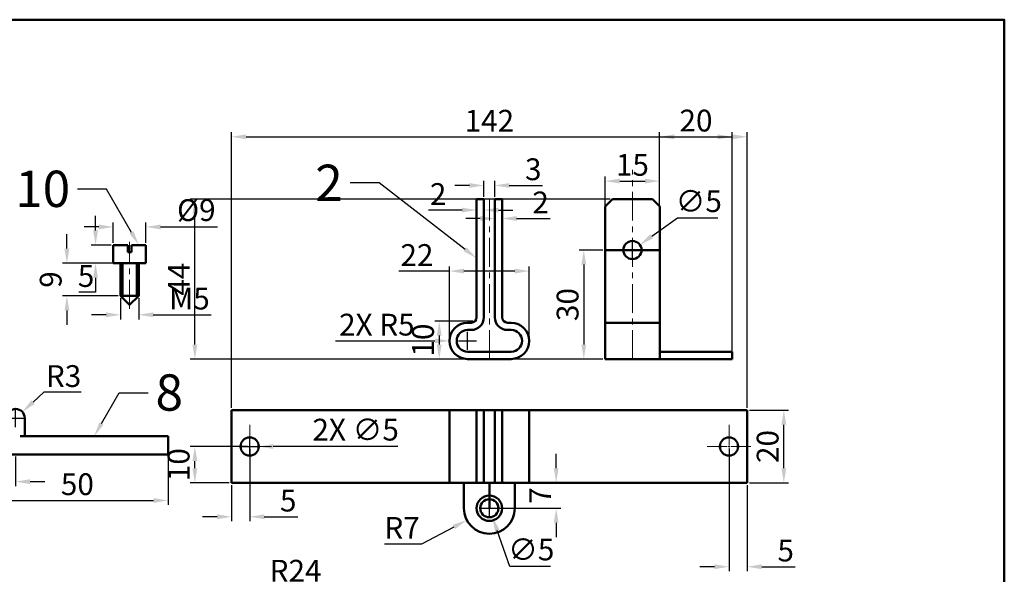
# Model space of a CAD drawing. Units: millimetres. Extents: x 1145 to 1687, y 12 to 400.
# Tile 6 of 6: x 1416 to 1687, y 247 to 400. Entities that reach past the tile are written whole.
import ezdxf
from ezdxf import colors
from ezdxf.entities.mleader import LeaderData, LeaderLine
from ezdxf.math import Vec2, Vec3

# ---------------------------------------------------------------- set-up
doc = ezdxf.new("R2010")
doc.units = ezdxf.units.MM
doc.header["$LTSCALE"] = 0.5
doc.linetypes.add('CENTER', pattern=[50.8, 31.75, -6.35, 6.35, -6.35])
for name, color, linetype, lineweight in [('M-CNTR', 1, 'CENTER', 18), ('M-DIMS', 2, 'Continuous', 25), ('M-OUTL', 7, 'Continuous', 50), ('M-TEXT', 3, 'Continuous', 25)]:
    doc.layers.add(name, color=color, linetype=linetype, lineweight=lineweight)
doc.styles.get("Standard").update_dxf_attribs({"font": 'arial.ttf'})
doc.dimstyles.new('ISO-25', dxfattribs={"dimtxt": 6, "dimasz": 4, "dimexe": 1.25, "dimexo": 0.625, "dimtad": 1, "dimtoh": 1, "dimdec": 0, "dimtxsty": 'Standard', "dimcen": 2.5, "dimadec": 0, "dimazin": 0, "dimtfac": 1, "dimtdec": 0, "dimtofl": 0, "dimtmove": 0, "dimatfit": 3, "dimfxl": 1, "dimarcsym": 0})

# ---------------------------------------------------------------- blocks, each defined once
blk = doc.blocks.new('*D22')
at = {"layer": 'Defpoints', "color": 0, "ltscale": 0.5, "transparency": 16777216}
for p in [(1450.76, 343.09), (1441.76, 338.11), (1450.76, 338.11)]:
    blk.add_point(p, dxfattribs=at)
at = {"layer": 'M-DIMS', "color": 0, "lineweight": -2, "ltscale": 0.5, "transparency": 16777216}
for p, q in [((1437.76, 343.09), (1433.76, 343.09)), ((1441.76, 338.74), (1441.76, 344.34)), ((1450.76, 338.74), (1450.76, 344.34)), ((1454.76, 343.09), (1470.48, 343.09))]:
    blk.add_line(p, q, dxfattribs=at)
at = {"layer": 'M-DIMS', "color": 0, "ltscale": 0.5, "transparency": 16777216}
for points in [[(1437.76, 343.76), (1437.76, 342.42), (1441.76, 343.09)], [(1454.76, 343.76), (1454.76, 342.42), (1450.76, 343.09)]]:
    blk.add_solid(points, dxfattribs=at)
at = {"layer": 'M-DIMS', "color": 0, "ltscale": 0.5, "transparency": 16777216, "insert": (1464.62, 346.94), "char_height": 6, "attachment_point": 5}
blk.add_mtext('%%C9', dxfattribs=at)
blk = doc.blocks.new('*D23')
at = {"layer": 'Defpoints', "color": 0, "ltscale": 0.5, "transparency": 16777216}
for p in [(1441.76, 338.11), (1436.87, 333.11), (1441.76, 333.11)]:
    blk.add_point(p, dxfattribs=at)
at = {"layer": 'M-DIMS', "color": 0, "lineweight": -2, "ltscale": 0.5, "transparency": 16777216}
for p, q in [((1436.87, 342.11), (1436.87, 346.11)), ((1441.14, 338.11), (1435.62, 338.11)), ((1441.14, 333.11), (1435.62, 333.11)), ((1436.87, 329.11), (1436.87, 325.11)), ((1436.87, 325.11), (1432.27, 325.11))]:
    blk.add_line(p, q, dxfattribs=at)
at = {"layer": 'M-DIMS', "color": 0, "ltscale": 0.5, "transparency": 16777216}
for points in [[(1436.2, 342.11), (1437.54, 342.11), (1436.87, 338.11)], [(1436.2, 329.11), (1437.54, 329.11), (1436.87, 333.11)]]:
    blk.add_solid(points, dxfattribs=at)
at = {"layer": 'M-DIMS', "color": 0, "ltscale": 0.5, "transparency": 16777216, "insert": (1434.26, 328.79), "char_height": 6, "attachment_point": 5}
blk.add_mtext('5', dxfattribs=at)
blk = doc.blocks.new('*D24')
at = {"layer": 'Defpoints', "color": 0, "ltscale": 0.5, "transparency": 16777216}
for p in [(1443.76, 324.11), (1448.76, 324.11), (1448.76, 318.9)]:
    blk.add_point(p, dxfattribs=at)
at = {"layer": 'M-DIMS', "color": 0, "lineweight": -2, "ltscale": 0.5, "transparency": 16777216}
for p, q in [((1443.76, 323.49), (1443.76, 317.65)), ((1448.76, 323.49), (1448.76, 317.65)), ((1439.76, 318.9), (1435.76, 318.9)), ((1452.76, 318.9), (1468.7, 318.9))]:
    blk.add_line(p, q, dxfattribs=at)
at = {"layer": 'M-DIMS', "color": 0, "ltscale": 0.5, "transparency": 16777216}
for points in [[(1439.76, 319.57), (1439.76, 318.24), (1443.76, 318.9)], [(1452.76, 319.57), (1452.76, 318.24), (1448.76, 318.9)]]:
    blk.add_solid(points, dxfattribs=at)
at = {"layer": 'M-DIMS', "color": 0, "ltscale": 0.5, "transparency": 16777216, "insert": (1462.73, 322.58), "char_height": 6, "attachment_point": 5}
blk.add_mtext('M5', dxfattribs=at)
blk = doc.blocks.new('*D25')
at = {"layer": 'Defpoints', "color": 0, "ltscale": 0.5, "transparency": 16777216}
for p in [(1443.76, 333.11), (1428.98, 324.11), (1443.76, 324.11)]:
    blk.add_point(p, dxfattribs=at)
at = {"layer": 'M-DIMS', "color": 0, "lineweight": -2, "ltscale": 0.5, "transparency": 16777216}
for p, q in [((1428.98, 337.11), (1428.98, 341.11)), ((1443.14, 333.11), (1427.73, 333.11)), ((1443.14, 324.11), (1427.73, 324.11)), ((1428.98, 320.11), (1428.98, 316.11))]:
    blk.add_line(p, q, dxfattribs=at)
at = {"layer": 'M-DIMS', "color": 0, "ltscale": 0.5, "transparency": 16777216}
for points in [[(1428.31, 337.11), (1429.65, 337.11), (1428.98, 333.11)], [(1428.31, 320.11), (1429.65, 320.11), (1428.98, 324.11)]]:
    blk.add_solid(points, dxfattribs=at)
at = {"layer": 'M-DIMS', "color": 0, "ltscale": 0.5, "transparency": 16777216, "insert": (1425.29, 328.61), "char_height": 6, "attachment_point": 5, "rotation": 90}
blk.add_mtext('9', dxfattribs=at)
blk = doc.blocks.new('*D41')
at = {"layer": 'Defpoints', "color": 0, "ltscale": 0.5, "transparency": 16777216}
for p in [(1406.86, 280.47), (1456.86, 280.47), (1456.86, 267.79)]:
    blk.add_point(p, dxfattribs=at)
at = {"layer": 'M-DIMS', "color": 0, "lineweight": -2, "ltscale": 0.5, "transparency": 16777216}
for p, q in [((1406.86, 279.85), (1406.86, 266.54)), ((1456.86, 279.85), (1456.86, 266.54)), ((1410.86, 267.79), (1452.86, 267.79))]:
    blk.add_line(p, q, dxfattribs=at)
at = {"layer": 'M-DIMS', "color": 0, "ltscale": 0.5, "transparency": 16777216}
for points in [[(1410.86, 268.45), (1410.86, 267.12), (1406.86, 267.79)], [(1452.86, 268.45), (1452.86, 267.12), (1456.86, 267.79)]]:
    blk.add_solid(points, dxfattribs=at)
at = {"layer": 'M-DIMS', "color": 0, "ltscale": 0.5, "transparency": 16777216, "insert": (1431.86, 271.48), "char_height": 6, "attachment_point": 5}
blk.add_mtext('50', dxfattribs=at)
blk = doc.blocks.new('*D42')
at = {"layer": 'Defpoints', "color": 0, "ltscale": 0.5, "transparency": 16777216}
for p in [(1406.86, 280.47), (1414.86, 280.47), (1414.86, 272.97)]:
    blk.add_point(p, dxfattribs=at)
at = {"layer": 'M-DIMS', "color": 0, "lineweight": -2, "ltscale": 0.5, "transparency": 16777216}
for p, q in [((1406.86, 279.85), (1406.86, 271.72)), ((1414.86, 279.85), (1414.86, 271.72)), ((1402.86, 272.97), (1398.86, 272.97)), ((1418.86, 272.97), (1422.86, 272.97))]:
    blk.add_line(p, q, dxfattribs=at)
at = {"layer": 'M-DIMS', "color": 0, "ltscale": 0.5, "transparency": 16777216}
for points in [[(1402.86, 273.63), (1402.86, 272.3), (1406.86, 272.97)], [(1418.86, 273.63), (1418.86, 272.3), (1414.86, 272.97)]]:
    blk.add_solid(points, dxfattribs=at)
at = {"layer": 'M-DIMS', "color": 0, "ltscale": 0.5, "transparency": 16777216, "insert": (1410.86, 276.66), "char_height": 6, "attachment_point": 5}
blk.add_mtext('8', dxfattribs=at)
blk = doc.blocks.new('*D45')
at = {"layer": 'Defpoints', "color": 0, "ltscale": 0.5, "transparency": 16777216}
for p in [(1546.82, 354.5), (1543.82, 350.72), (1546.82, 350.72)]:
    blk.add_point(p, dxfattribs=at)
at = {"layer": 'M-DIMS', "color": 0, "lineweight": -2, "ltscale": 0.5, "transparency": 16777216}
for p, q in [((1543.82, 351.35), (1543.82, 355.75)), ((1546.82, 351.35), (1546.82, 355.75)), ((1539.82, 354.5), (1535.82, 354.5)), ((1550.82, 354.5), (1560, 354.5))]:
    blk.add_line(p, q, dxfattribs=at)
at = {"layer": 'M-DIMS', "color": 0, "ltscale": 0.5, "transparency": 16777216}
for points in [[(1539.82, 355.17), (1539.82, 353.84), (1543.82, 354.5)], [(1550.82, 355.17), (1550.82, 353.84), (1546.82, 354.5)]]:
    blk.add_solid(points, dxfattribs=at)
at = {"layer": 'M-DIMS', "color": 0, "ltscale": 0.5, "transparency": 16777216, "insert": (1557.41, 358.19), "char_height": 6, "attachment_point": 5}
blk.add_mtext('3', dxfattribs=at)
blk = doc.blocks.new('*D46')
at = {"layer": 'Defpoints', "color": 0, "ltscale": 0.5, "transparency": 16777216}
for p in [(1546.82, 350.72), (1548.82, 350.72), (1548.82, 345.41)]:
    blk.add_point(p, dxfattribs=at)
at = {"layer": 'M-DIMS', "color": 0, "lineweight": -2, "ltscale": 0.5, "transparency": 16777216}
for p, q in [((1546.82, 350.1), (1546.82, 344.16)), ((1548.82, 350.1), (1548.82, 344.16)), ((1542.82, 345.41), (1538.82, 345.41)), ((1552.82, 345.41), (1562.04, 345.41))]:
    blk.add_line(p, q, dxfattribs=at)
at = {"layer": 'M-DIMS', "color": 0, "ltscale": 0.5, "transparency": 16777216}
for points in [[(1542.82, 346.08), (1542.82, 344.75), (1546.82, 345.41)], [(1552.82, 346.08), (1552.82, 344.75), (1548.82, 345.41)]]:
    blk.add_solid(points, dxfattribs=at)
at = {"layer": 'M-DIMS', "color": 0, "ltscale": 0.5, "transparency": 16777216, "insert": (1559.43, 349.05), "char_height": 6, "attachment_point": 5}
blk.add_mtext('2', dxfattribs=at)
blk = doc.blocks.new('*D47')
at = {"layer": 'Defpoints', "color": 0, "ltscale": 0.5, "transparency": 16777216}
for p in [(1541.82, 350.72), (1543.82, 350.72), (1543.82, 347.73)]:
    blk.add_point(p, dxfattribs=at)
at = {"layer": 'M-DIMS', "color": 0, "lineweight": -2, "ltscale": 0.5, "transparency": 16777216}
for p, q in [((1541.82, 350.1), (1541.82, 346.48)), ((1543.82, 350.1), (1543.82, 346.48)), ((1537.82, 347.73), (1528.6, 347.73)), ((1547.82, 347.73), (1551.82, 347.73))]:
    blk.add_line(p, q, dxfattribs=at)
at = {"layer": 'M-DIMS', "color": 0, "ltscale": 0.5, "transparency": 16777216}
for points in [[(1537.82, 348.39), (1537.82, 347.06), (1541.82, 347.73)], [(1547.82, 348.39), (1547.82, 347.06), (1543.82, 347.73)]]:
    blk.add_solid(points, dxfattribs=at)
at = {"layer": 'M-DIMS', "color": 0, "ltscale": 0.5, "transparency": 16777216, "insert": (1531.21, 351.36), "char_height": 6, "attachment_point": 5}
blk.add_mtext('2', dxfattribs=at)
blk = doc.blocks.new('*D48')
at = {"layer": 'Defpoints', "color": 0, "ltscale": 0.5, "transparency": 16777216}
for p in [(1577.22, 336.72), (1571.33, 306.72), (1577.22, 306.72)]:
    blk.add_point(p, dxfattribs=at)
at = {"layer": 'M-DIMS', "color": 0, "lineweight": -2, "ltscale": 0.5, "transparency": 16777216}
for p, q in [((1576.6, 336.72), (1570.08, 336.72)), ((1571.33, 332.72), (1571.33, 310.72)), ((1576.6, 306.72), (1570.08, 306.72))]:
    blk.add_line(p, q, dxfattribs=at)
at = {"layer": 'M-DIMS', "color": 0, "ltscale": 0.5, "transparency": 16777216}
for points in [[(1570.66, 332.72), (1571.99, 332.72), (1571.33, 336.72)], [(1570.66, 310.72), (1571.99, 310.72), (1571.33, 306.72)]]:
    blk.add_solid(points, dxfattribs=at)
at = {"layer": 'M-DIMS', "color": 0, "ltscale": 0.5, "transparency": 16777216, "insert": (1567.64, 321.72), "char_height": 6, "attachment_point": 5, "rotation": 90}
blk.add_mtext('30', dxfattribs=at)
blk = doc.blocks.new('*D49')
at = {"layer": 'Defpoints', "color": 0, "ltscale": 0.5, "transparency": 16777216}
for p in [(1541.38, 317.16), (1531.52, 306.72), (1541.38, 306.72)]:
    blk.add_point(p, dxfattribs=at)
at = {"layer": 'M-DIMS', "color": 0, "lineweight": -2, "ltscale": 0.5, "transparency": 16777216}
for p, q in [((1540.76, 317.16), (1530.27, 317.16)), ((1531.52, 313.16), (1531.52, 310.72)), ((1540.76, 306.72), (1530.27, 306.72))]:
    blk.add_line(p, q, dxfattribs=at)
at = {"layer": 'M-DIMS', "color": 0, "ltscale": 0.5, "transparency": 16777216}
for points in [[(1530.85, 313.16), (1532.19, 313.16), (1531.52, 317.16)], [(1530.85, 310.72), (1532.19, 310.72), (1531.52, 306.72)]]:
    blk.add_solid(points, dxfattribs=at)
at = {"layer": 'M-DIMS', "color": 0, "ltscale": 0.5, "transparency": 16777216, "insert": (1527.83, 311.94), "char_height": 6, "attachment_point": 5, "rotation": 90}
blk.add_mtext('10', dxfattribs=at)
blk = doc.blocks.new('*D50')
at = {"layer": 'Defpoints', "color": 0, "ltscale": 0.5, "transparency": 16777216}
for p in [(1556.32, 330.94), (1534.32, 311.72), (1556.32, 311.72)]:
    blk.add_point(p, dxfattribs=at)
at = {"layer": 'M-DIMS', "color": 0, "lineweight": -2, "ltscale": 0.5, "transparency": 16777216}
for p, q in [((1534.32, 330.94), (1520.43, 330.94)), ((1534.32, 312.35), (1534.32, 332.19)), ((1552.32, 330.94), (1538.32, 330.94)), ((1556.32, 312.35), (1556.32, 332.19))]:
    blk.add_line(p, q, dxfattribs=at)
at = {"layer": 'M-DIMS', "color": 0, "ltscale": 0.5, "transparency": 16777216}
for points in [[(1538.32, 331.6), (1538.32, 330.27), (1534.32, 330.94)], [(1552.32, 331.6), (1552.32, 330.27), (1556.32, 330.94)]]:
    blk.add_solid(points, dxfattribs=at)
at = {"layer": 'M-DIMS', "color": 0, "ltscale": 0.5, "transparency": 16777216, "insert": (1525.38, 334.57), "char_height": 6, "attachment_point": 5}
blk.add_mtext('22', dxfattribs=at)
blk = doc.blocks.new('*D51')
at = {"layer": 'Defpoints', "color": 0, "ltscale": 0.5, "transparency": 16777216}
for p in [(1592.22, 355.71), (1577.22, 342.72), (1592.22, 342.72)]:
    blk.add_point(p, dxfattribs=at)
at = {"layer": 'M-DIMS', "color": 0, "lineweight": -2, "ltscale": 0.5, "transparency": 16777216}
for p, q in [((1577.22, 343.35), (1577.22, 356.96)), ((1581.22, 355.71), (1588.22, 355.71)), ((1592.22, 343.35), (1592.22, 356.96))]:
    blk.add_line(p, q, dxfattribs=at)
at = {"layer": 'M-DIMS', "color": 0, "ltscale": 0.5, "transparency": 16777216}
for points in [[(1581.22, 356.38), (1581.22, 355.05), (1577.22, 355.71)], [(1588.22, 356.38), (1588.22, 355.05), (1592.22, 355.71)]]:
    blk.add_solid(points, dxfattribs=at)
at = {"layer": 'M-DIMS', "color": 0, "ltscale": 0.5, "transparency": 16777216, "insert": (1584.72, 359.4), "char_height": 6, "attachment_point": 5}
blk.add_mtext('15', dxfattribs=at)
blk = doc.blocks.new('*D52')
at = {"layer": 'Defpoints', "color": 0, "ltscale": 0.5, "transparency": 16777216}
for p in [(1586.76, 338.17), (1582.69, 335.27)]:
    blk.add_point(p, dxfattribs=at)
at = {"layer": 'M-DIMS', "color": 0, "lineweight": -2, "ltscale": 0.5, "transparency": 16777216}
for p, q in [((1597.11, 345.54), (1590.02, 340.49)), ((1608.24, 345.54), (1597.11, 345.54)), ((1584.72, 334.22), (1584.72, 339.22)), ((1582.22, 336.72), (1587.22, 336.72))]:
    blk.add_line(p, q, dxfattribs=at)
at = {"layer": 'M-DIMS', "color": 0, "ltscale": 0.5, "transparency": 16777216}
blk.add_solid([(1589.63, 341.04), (1590.4, 339.95), (1586.76, 338.17)], dxfattribs=at)
at = {"layer": 'M-DIMS', "color": 0, "ltscale": 0.5, "transparency": 16777216, "insert": (1602.99, 349.4), "char_height": 6, "attachment_point": 5}
blk.add_mtext('∅5', dxfattribs=at)
blk = doc.blocks.new('*U56')
at = {"layer": 'M-CNTR', "color": 0, "transparency": 16777216}
for p, q in [((0, 0.5), (0, 6)), ((-6, 0), (-0.5, 0)), ((0.5, 0), (6, 0)), ((0, -6), (0, -0.5))]:
    blk.add_line(p, q, dxfattribs=at)
at = {"layer": 'M-CNTR', "color": 0, "linetype": 'Continuous', "transparency": 16777216}
for p, q in [((-0.25, 0), (0.25, 0)), ((0, -0.25), (0, 0.25))]:
    blk.add_line(p, q, dxfattribs=at)
blk = doc.blocks.new('*U57')
at = {"layer": 'M-CNTR', "color": 0, "transparency": 16777216}
for p, q in [((0, 0.5), (0, 6)), ((-6, 0), (-0.5, 0)), ((0.5, 0), (6, 0)), ((0, -6), (0, -0.5))]:
    blk.add_line(p, q, dxfattribs=at)
at = {"layer": 'M-CNTR', "color": 0, "linetype": 'Continuous', "transparency": 16777216}
for p, q in [((-0.25, 0), (0.25, 0)), ((0, -0.25), (0, 0.25))]:
    blk.add_line(p, q, dxfattribs=at)
blk = doc.blocks.new('*D58')
at = {"layer": 'Defpoints', "color": 0, "ltscale": 0.5, "transparency": 16777216}
for p in [(1479.32, 282.64), (1474.32, 272.64), (1479.32, 263.29)]:
    blk.add_point(p, dxfattribs=at)
at = {"layer": 'M-DIMS', "color": 0, "lineweight": -2, "ltscale": 0.5, "transparency": 16777216}
for p, q in [((1479.32, 282.02), (1479.32, 262.04)), ((1474.32, 272.02), (1474.32, 262.04)), ((1470.32, 263.29), (1466.32, 263.29)), ((1483.32, 263.29), (1492.55, 263.29))]:
    blk.add_line(p, q, dxfattribs=at)
at = {"layer": 'M-DIMS', "color": 0, "ltscale": 0.5, "transparency": 16777216}
for points in [[(1470.32, 263.96), (1470.32, 262.62), (1474.32, 263.29)], [(1483.32, 263.96), (1483.32, 262.62), (1479.32, 263.29)]]:
    blk.add_solid(points, dxfattribs=at)
at = {"layer": 'M-DIMS', "color": 0, "ltscale": 0.5, "transparency": 16777216, "insert": (1489.93, 266.97), "char_height": 6, "attachment_point": 5}
blk.add_mtext('5', dxfattribs=at)
blk = doc.blocks.new('*D59')
at = {"layer": 'Defpoints', "color": 0, "ltscale": 0.5, "transparency": 16777216}
for p in [(1414.86, 290.47), (1416.7, 292.16)]:
    blk.add_point(p, dxfattribs=at)
at = {"layer": 'M-DIMS', "color": 0, "lineweight": -2, "ltscale": 0.5, "transparency": 16777216}
for p, q in [((1422.6, 297.56), (1419.65, 294.86)), ((1432.9, 297.56), (1422.6, 297.56)), ((1414.86, 287.97), (1414.86, 292.97)), ((1412.36, 290.47), (1417.36, 290.47))]:
    blk.add_line(p, q, dxfattribs=at)
at = {"layer": 'M-DIMS', "color": 0, "ltscale": 0.5, "transparency": 16777216}
blk.add_solid([(1419.2, 295.35), (1420.1, 294.37), (1416.7, 292.16)], dxfattribs=at)
at = {"layer": 'M-DIMS', "color": 0, "ltscale": 0.5, "transparency": 16777216, "insert": (1428.06, 301.25), "char_height": 6, "attachment_point": 5}
blk.add_mtext('R3', dxfattribs=at)
blk = doc.blocks.new('*D66')
at = {"layer": 'Defpoints', "color": 0, "ltscale": 0.5, "transparency": 16777216}
for p in [(1545.32, 272.64), (1545.32, 265.64), (1563.72, 265.64)]:
    blk.add_point(p, dxfattribs=at)
at = {"layer": 'M-DIMS', "color": 0, "lineweight": -2, "ltscale": 0.5, "transparency": 16777216}
for p, q in [((1563.72, 276.64), (1563.72, 280.64)), ((1545.95, 272.64), (1564.97, 272.64)), ((1545.95, 265.64), (1564.97, 265.64)), ((1563.72, 261.64), (1563.72, 257.64))]:
    blk.add_line(p, q, dxfattribs=at)
at = {"layer": 'M-DIMS', "color": 0, "ltscale": 0.5, "transparency": 16777216}
for points in [[(1563.05, 276.64), (1564.38, 276.64), (1563.72, 272.64)], [(1563.05, 261.64), (1564.38, 261.64), (1563.72, 265.64)]]:
    blk.add_solid(points, dxfattribs=at)
at = {"layer": 'M-DIMS', "color": 0, "ltscale": 0.5, "transparency": 16777216, "insert": (1560.09, 269.14), "char_height": 6, "attachment_point": 5, "rotation": 90}
blk.add_mtext('7', dxfattribs=at)
blk = doc.blocks.new('*D67')
at = {"layer": 'Defpoints', "color": 0, "ltscale": 0.5, "transparency": 16777216}
for p in [(1545.32, 265.64), (1539.13, 262.37)]:
    blk.add_point(p, dxfattribs=at)
at = {"layer": 'M-DIMS', "color": 0, "lineweight": -2, "ltscale": 0.5, "transparency": 16777216}
for p, q in [((1545.32, 263.14), (1545.32, 268.14)), ((1542.82, 265.64), (1547.82, 265.64)), ((1526.75, 255.84), (1535.59, 260.51)), ((1516.45, 255.84), (1526.75, 255.84))]:
    blk.add_line(p, q, dxfattribs=at)
at = {"layer": 'M-DIMS', "color": 0, "ltscale": 0.5, "transparency": 16777216}
blk.add_solid([(1535.28, 261.09), (1535.9, 259.92), (1539.13, 262.37)], dxfattribs=at)
at = {"layer": 'M-DIMS', "color": 0, "ltscale": 0.5, "transparency": 16777216, "insert": (1521.29, 259.46), "char_height": 6, "attachment_point": 5}
blk.add_mtext('R7', dxfattribs=at)
blk = doc.blocks.new('*D68')
at = {"layer": 'Defpoints', "color": 0, "ltscale": 0.5, "transparency": 16777216}
for p in [(1544.49, 268), (1546.16, 263.28)]:
    blk.add_point(p, dxfattribs=at)
at = {"layer": 'M-DIMS', "color": 0, "lineweight": -2, "ltscale": 0.5, "transparency": 16777216}
for p, q in [((1545.32, 263.14), (1545.32, 268.14)), ((1542.82, 265.64), (1547.82, 265.64)), ((1550.99, 249.65), (1547.49, 259.51)), ((1562.12, 249.65), (1550.99, 249.65))]:
    blk.add_line(p, q, dxfattribs=at)
at = {"layer": 'M-DIMS', "color": 0, "ltscale": 0.5, "transparency": 16777216}
blk.add_solid([(1548.12, 259.74), (1546.86, 259.29), (1546.16, 263.28)], dxfattribs=at)
at = {"layer": 'M-DIMS', "color": 0, "ltscale": 0.5, "transparency": 16777216, "insert": (1556.86, 253.51), "char_height": 6, "attachment_point": 5}
blk.add_mtext('∅5', dxfattribs=at)
blk = doc.blocks.new('CONTACT-CLIP')
at = {"ltscale": 0.5}
for p, q in [((7.5, 11.5), (7.5, 44)), ((7.5, 44), (9.5, 44)), ((9.5, 11.5), (9.5, 44)), ((12.5, 11.5), (12.5, 44)), ((12.5, 44), (14.5, 44)), ((14.5, 11.5), (14.5, 44)), ((5, 10), (6, 10)), ((5, 2), (17, 2)), ((5, 0), (17, 0))]:
    blk.add_line(p, q, dxfattribs=at)
for centre, radius, start, end in [((6, 11.5), 1.5, 270, 0), ((6, 11.5), 3.5, 270, 0), ((16, 11.5), 3.5, 180, 270), ((16, 11.5), 1.5, 180, 270), ((5, 5), 5, 90, 270), ((17, 5), 5, 270, 90), ((5, 5), 3, 90, 270), ((17, 5), 3, 270, 90)]:
    blk.add_arc(centre, radius, start, end, dxfattribs=at)
for points in [[(16, 10), (16.33, 10), (16.67, 10), (17, 10)], [(6, 8), (5.67, 8), (5.33, 8), (5, 8)], [(16, 8), (16.33, 8), (16.67, 8), (17, 8)]]:
    blk.add_open_spline(points, degree=3)
blk = doc.blocks.new('SCREW-HEAD')
at = {"ltscale": 0.5}
for p, q in [((0, 5), (4, 5)), ((0, 0), (0, 5)), ((4, 5), (4, 3)), ((4, 3), (5, 3)), ((5, 5), (5, 3)), ((5, 5), (9, 5)), ((9, 5), (9, 0)), ((9, 0), (0, 0))]:
    blk.add_line(p, q, dxfattribs=at)
blk = doc.blocks.new('TERMINAL-LUG-END')
at = {"ltscale": 0.5}
for p, q in [((0, 7), (0, 14)), ((14, 7), (14, 14))]:
    blk.add_line(p, q, dxfattribs=at)
blk.add_arc((7, 7), 7, 180, 0, dxfattribs=at)
blk = doc.blocks.new('*D90')
at = {"layer": 'Defpoints', "color": 0, "ltscale": 0.5, "transparency": 16777216}
for p in [(1616.32, 367.9), (1474.32, 292.64), (1616.32, 292.64)]:
    blk.add_point(p, dxfattribs=at)
at = {"layer": 'M-DIMS', "color": 0, "lineweight": -2, "ltscale": 0.5, "transparency": 16777216}
for p, q in [((1474.32, 293.27), (1474.32, 369.15)), ((1616.32, 293.27), (1616.32, 369.15)), ((1478.32, 367.9), (1612.32, 367.9))]:
    blk.add_line(p, q, dxfattribs=at)
at = {"layer": 'M-DIMS', "color": 0, "ltscale": 0.5, "transparency": 16777216}
for points in [[(1478.32, 368.57), (1478.32, 367.23), (1474.32, 367.9)], [(1612.32, 368.57), (1612.32, 367.23), (1616.32, 367.9)]]:
    blk.add_solid(points, dxfattribs=at)
at = {"layer": 'M-DIMS', "color": 0, "ltscale": 0.5, "transparency": 16777216, "insert": (1545.32, 371.54), "char_height": 6, "attachment_point": 5}
blk.add_mtext('142', dxfattribs=at)
blk = doc.blocks.new('*D91')
at = {"layer": 'Defpoints', "color": 0, "ltscale": 0.5, "transparency": 16777216}
for p in [(1616.32, 292.64), (1626.42, 292.64), (1616.32, 272.64)]:
    blk.add_point(p, dxfattribs=at)
at = {"layer": 'M-DIMS', "color": 0, "lineweight": -2, "ltscale": 0.5, "transparency": 16777216}
for p, q in [((1616.95, 292.64), (1627.67, 292.64)), ((1626.42, 276.64), (1626.42, 288.64)), ((1616.95, 272.64), (1627.67, 272.64))]:
    blk.add_line(p, q, dxfattribs=at)
at = {"layer": 'M-DIMS', "color": 0, "ltscale": 0.5, "transparency": 16777216}
for points in [[(1625.75, 288.64), (1627.09, 288.64), (1626.42, 292.64)], [(1625.75, 276.64), (1627.09, 276.64), (1626.42, 272.64)]]:
    blk.add_solid(points, dxfattribs=at)
at = {"layer": 'M-DIMS', "color": 0, "ltscale": 0.5, "transparency": 16777216, "insert": (1622.73, 282.64), "char_height": 6, "attachment_point": 5, "rotation": 90}
blk.add_mtext('20', dxfattribs=at)
blk = doc.blocks.new('*D92')
at = {"layer": 'Defpoints', "color": 0, "ltscale": 0.5, "transparency": 16777216}
for p in [(1611.32, 282.64), (1616.32, 272.64), (1616.32, 249.54)]:
    blk.add_point(p, dxfattribs=at)
at = {"layer": 'M-DIMS', "color": 0, "lineweight": -2, "ltscale": 0.5, "transparency": 16777216}
for p, q in [((1611.32, 282.02), (1611.32, 248.29)), ((1616.32, 272.02), (1616.32, 248.29)), ((1607.32, 249.54), (1603.32, 249.54)), ((1620.32, 249.54), (1629.55, 249.54))]:
    blk.add_line(p, q, dxfattribs=at)
at = {"layer": 'M-DIMS', "color": 0, "ltscale": 0.5, "transparency": 16777216}
for points in [[(1607.32, 250.21), (1607.32, 248.87), (1611.32, 249.54)], [(1620.32, 250.21), (1620.32, 248.87), (1616.32, 249.54)]]:
    blk.add_solid(points, dxfattribs=at)
at = {"layer": 'M-DIMS', "color": 0, "ltscale": 0.5, "transparency": 16777216, "insert": (1626.93, 253.22), "char_height": 6, "attachment_point": 5}
blk.add_mtext('5', dxfattribs=at)
blk = doc.blocks.new('*D93')
at = {"layer": 'Defpoints', "color": 0, "ltscale": 0.5, "transparency": 16777216}
for p in [(1464.22, 282.64), (1479.32, 282.64), (1474.32, 272.64)]:
    blk.add_point(p, dxfattribs=at)
at = {"layer": 'M-DIMS', "color": 0, "lineweight": -2, "ltscale": 0.5, "transparency": 16777216}
for p, q in [((1478.7, 282.64), (1462.97, 282.64)), ((1464.22, 276.64), (1464.22, 278.64)), ((1473.7, 272.64), (1462.97, 272.64))]:
    blk.add_line(p, q, dxfattribs=at)
at = {"layer": 'M-DIMS', "color": 0, "ltscale": 0.5, "transparency": 16777216}
for points in [[(1463.55, 278.64), (1464.89, 278.64), (1464.22, 282.64)], [(1463.55, 276.64), (1464.89, 276.64), (1464.22, 272.64)]]:
    blk.add_solid(points, dxfattribs=at)
at = {"layer": 'M-DIMS', "color": 0, "ltscale": 0.5, "transparency": 16777216, "insert": (1460.53, 277.64), "char_height": 6, "attachment_point": 5, "rotation": 90}
blk.add_mtext('10', dxfattribs=at)
blk = doc.blocks.new('*D94')
at = {"layer": 'Defpoints', "color": 0, "ltscale": 0.5, "transparency": 16777216}
for p in [(1464.22, 350.72), (1579.22, 350.72), (1577.22, 306.72)]:
    blk.add_point(p, dxfattribs=at)
at = {"layer": 'M-DIMS', "color": 0, "lineweight": -2, "ltscale": 0.5, "transparency": 16777216}
for p, q in [((1578.6, 350.72), (1462.97, 350.72)), ((1464.22, 310.72), (1464.22, 346.72)), ((1576.6, 306.72), (1462.97, 306.72))]:
    blk.add_line(p, q, dxfattribs=at)
at = {"layer": 'M-DIMS', "color": 0, "ltscale": 0.5, "transparency": 16777216}
for points in [[(1463.55, 346.72), (1464.89, 346.72), (1464.22, 350.72)], [(1463.55, 310.72), (1464.89, 310.72), (1464.22, 306.72)]]:
    blk.add_solid(points, dxfattribs=at)
at = {"layer": 'M-DIMS', "color": 0, "ltscale": 0.5, "transparency": 16777216, "insert": (1460.6, 328.72), "char_height": 6, "attachment_point": 5, "rotation": 90}
blk.add_mtext('44', dxfattribs=at)
blk = doc.blocks.new('*D95')
at = {"layer": 'Defpoints', "color": 0, "ltscale": 0.5, "transparency": 16777216}
for p in [(1612.22, 367.9), (1592.22, 306.72), (1612.22, 306.72)]:
    blk.add_point(p, dxfattribs=at)
at = {"layer": 'M-DIMS', "color": 0, "lineweight": -2, "ltscale": 0.5, "transparency": 16777216}
for p, q in [((1592.22, 307.35), (1592.22, 369.15)), ((1612.22, 307.35), (1612.22, 369.15)), ((1596.22, 367.9), (1608.22, 367.9))]:
    blk.add_line(p, q, dxfattribs=at)
at = {"layer": 'M-DIMS', "color": 0, "ltscale": 0.5, "transparency": 16777216}
for points in [[(1596.22, 368.57), (1596.22, 367.23), (1592.22, 367.9)], [(1608.22, 368.57), (1608.22, 367.23), (1612.22, 367.9)]]:
    blk.add_solid(points, dxfattribs=at)
at = {"layer": 'M-DIMS', "color": 0, "ltscale": 0.5, "transparency": 16777216, "insert": (1602.22, 371.59), "char_height": 6, "attachment_point": 5}
blk.add_mtext('20', dxfattribs=at)
blk = doc.blocks.new('*D115')
at = {"layer": 'Defpoints', "color": 0, "ltscale": 0.5, "transparency": 16777216}
for p in [(1476.82, 282.64), (1481.82, 282.64)]:
    blk.add_point(p, dxfattribs=at)
at = {"layer": 'M-DIMS', "color": 0, "lineweight": -2, "ltscale": 0.5, "transparency": 16777216}
for p, q in [((1479.32, 280.14), (1479.32, 285.14)), ((1476.82, 282.64), (1481.82, 282.64)), ((1496.28, 282.64), (1485.82, 282.64)), ((1520.09, 282.64), (1496.28, 282.64))]:
    blk.add_line(p, q, dxfattribs=at)
at = {"layer": 'M-DIMS', "color": 0, "ltscale": 0.5, "transparency": 16777216}
blk.add_solid([(1485.82, 283.31), (1485.82, 281.97), (1481.82, 282.64)], dxfattribs=at)
at = {"layer": 'M-DIMS', "color": 0, "ltscale": 0.5, "transparency": 16777216, "insert": (1508.5, 286.5), "char_height": 6, "attachment_point": 5}
blk.add_mtext('2X ∅5', dxfattribs=at)
blk = doc.blocks.new('*D116')
at = {"layer": 'Defpoints', "color": 0, "ltscale": 0.5, "transparency": 16777216}
for p in [(1534.32, 311.72), (1539.32, 311.72)]:
    blk.add_point(p, dxfattribs=at)
at = {"layer": 'M-DIMS', "color": 0, "lineweight": -2, "ltscale": 0.5, "transparency": 16777216}
for p, q in [((1539.32, 309.22), (1539.32, 314.22)), ((1502.98, 311.72), (1526.32, 311.72)), ((1526.32, 311.72), (1530.32, 311.72)), ((1536.82, 311.72), (1541.82, 311.72))]:
    blk.add_line(p, q, dxfattribs=at)
at = {"layer": 'M-DIMS', "color": 0, "ltscale": 0.5, "transparency": 16777216}
blk.add_solid([(1530.32, 312.39), (1530.32, 311.06), (1534.32, 311.72)], dxfattribs=at)
at = {"layer": 'M-DIMS', "color": 0, "ltscale": 0.5, "transparency": 16777216, "insert": (1514.34, 315.41), "char_height": 6, "attachment_point": 5}
blk.add_mtext('2X R5', dxfattribs=at)
blk = doc.blocks.new('*D119')
at = {"layer": 'Defpoints', "color": 0, "ltscale": 0.5, "transparency": 16777216}
for p in [(1499.73, 229.62), (1499.73, 205.62)]:
    blk.add_point(p, dxfattribs=at)
at = {"layer": 'M-DIMS', "color": 0, "lineweight": -2, "ltscale": 0.5, "transparency": 16777216}
for p, q in [((1484.79, 244.02), (1499.73, 244.02)), ((1499.73, 244.02), (1499.73, 233.62)), ((1499.73, 203.12), (1499.73, 208.12)), ((1497.23, 205.62), (1502.23, 205.62))]:
    blk.add_line(p, q, dxfattribs=at)
at = {"layer": 'M-DIMS', "color": 0, "ltscale": 0.5, "transparency": 16777216}
blk.add_solid([(1500.4, 233.62), (1499.07, 233.62), (1499.73, 229.62)], dxfattribs=at)
at = {"layer": 'M-DIMS', "color": 0, "ltscale": 0.5, "transparency": 16777216, "insert": (1491.95, 247.66), "char_height": 6, "attachment_point": 5}
blk.add_mtext('R24', dxfattribs=at)

msp = doc.modelspace()

# ---------------------------------------------------------------- linework, layer by layer
at = {"layer": 'M-CNTR', "ltscale": 0.5}
for p, q in [((1584.7228, 306.7236), (1584.7228, 358.8009)), ((1545.3206, 306.7236), (1545.3206, 350.7236)), ((1446.2604, 320.5579), (1446.2604, 338.9798))]:
    msp.add_line(p, q, dxfattribs=at)
at = {"layer": 'M-OUTL', "ltscale": 0.5}
for p, q in [((1577.2228, 348.7236), (1579.2228, 350.7236)), ((1579.2228, 350.7236), (1590.2228, 350.7236)), ((1592.2228, 348.7236), (1590.2228, 350.7236)), ((1577.2228, 336.7236), (1577.2228, 348.7236)), ((1592.2228, 348.7236), (1592.2228, 336.7236)), ((1592.2228, 336.7236), (1577.2228, 336.7236)), ((1577.2228, 336.7236), (1577.2228, 306.7236)), ((1592.2228, 306.7236), (1592.2228, 336.7236)), ((1443.7604, 333.1137), (1443.7604, 324.1137)), ((1444.2604, 333.1137), (1444.2604, 324.1137)), ((1448.2604, 333.1137), (1448.2604, 324.1137)), ((1448.7604, 333.1137), (1448.7604, 324.1137)), ((1448.7604, 324.1137), (1443.7604, 324.1137)), ((1443.7604, 324.1137), (1446.2604, 321.6152)), ((1448.7604, 324.1137), (1446.2604, 321.6152)), ((1577.2228, 316.7236), (1592.2228, 316.7236)), ((1577.2228, 306.7236), (1592.2228, 306.7236)), ((1612.2228, 308.7236), (1592.2228, 308.7236)), ((1592.2228, 306.7236), (1612.2228, 306.7236)), ((1612.2228, 306.7236), (1612.2228, 308.7236)), ((1417.3568, 290.4724), (1417.3568, 285.4724)), ((1534.3206, 292.6401), (1474.3206, 292.6401)), ((1474.3206, 292.6401), (1474.3206, 272.6401)), ((1534.3206, 292.6401), (1534.3206, 272.6401)), ((1556.3206, 292.6401), (1534.3206, 292.6401)), ((1541.8206, 292.6401), (1541.8206, 272.6401)), ((1543.8206, 292.6401), (1543.8206, 272.6401)), ((1546.8206, 292.6401), (1546.8206, 272.6401)), ((1548.8206, 292.6401), (1548.8206, 272.6401)), ((1556.3206, 292.6401), (1556.3206, 272.6401)), ((1556.3206, 292.6401), (1616.3206, 292.6401)), ((1616.3206, 292.6401), (1616.3206, 272.6401)), ((1456.8568, 285.4724), (1416.1068, 285.4724)), ((1456.8568, 280.4724), (1456.8568, 285.4724)), ((1406.8568, 280.4724), (1456.8568, 280.4724)), ((1474.3206, 272.6401), (1534.3206, 272.6401)), ((1556.3206, 272.6401), (1534.3206, 272.6401)), ((1545.3206, 272.6401), (1545.3206, 265.6401)), ((1616.3206, 272.6401), (1556.3206, 272.6401))]:
    msp.add_line(p, q, dxfattribs=at)
msp.add_lwpolyline([(1145.3327, 400.1417), (1687.1285, 400.1417), (1687.1285, 12.2645), (1145.3327, 12.2645)], close=True, dxfattribs=at)
for centre, radius in [((1584.7228, 336.7236), 2.5), ((1479.3206, 282.6401), 2.5), ((1611.3206, 282.6401), 2.5), ((1545.3206, 265.6401), 3.5), ((1545.3206, 265.6401), 2.5)]:
    msp.add_circle(centre, radius, dxfattribs=at)
msp.add_arc((1414.8568, 290.4724), 2.5, 0, 180, dxfattribs=at)

# ---------------------------------------------------------------- block references
at = {"layer": 'M-CNTR'}
for name, p in [('*U57', (1479.3206, 282.6401)), ('*U56', (1611.3206, 282.6401))]:
    msp.add_blockref(name, p, dxfattribs=at)
at = {"layer": 'M-OUTL'}
for name, p in [('CONTACT-CLIP', (1534.321, 306.724)), ('SCREW-HEAD', (1441.76, 333.114)), ('TERMINAL-LUG-END', (1538.321, 258.64))]:
    msp.add_blockref(name, p, dxfattribs=at)

# ---------------------------------------------------------------- dimensions: what is measured, and where the dimension line sits
at = {"layer": 'M-DIMS', "ltscale": 0.5}
for base, p1, p2, override, picture, middle in [((1616.3206, 367.9009), (1474.3206, 292.6401), (1616.3206, 292.6401), {"dimdec": 0, "dimlfac": 1, "dimrnd": 0, "dimzin": 0, "dimdsep": 46, "dimlunit": 2}, '*D90', (1545.3206, 371.5382)), ((1612.2228, 367.9009), (1592.2228, 306.7236), (1612.2228, 306.7236), {"dimdec": 0, "dimlfac": 1, "dimrnd": 0, "dimzin": 0, "dimdsep": 46, "dimlunit": 2}, '*D95', (1602.2228, 371.5893)), ((1592.2228, 355.714), (1577.2228, 342.7236), (1592.2228, 342.7236), {"dimclrd": 0, "dimclre": 0, "dimclrt": 0}, '*D51', (1584.7228, 359.4024)), ((1546.8206, 354.5041), (1543.8206, 350.7236), (1546.8206, 350.7236), {"dimclrd": 0, "dimclre": 0, "dimclrt": 0}, '*D45', (1557.4101, 358.1946)), ((1548.8206, 345.4149), (1546.8206, 350.7236), (1548.8206, 350.7236), {"dimclrd": 0, "dimclre": 0, "dimclrt": 0}, '*D46', (1559.4326, 349.0522)), ((1479.3206, 263.2901), (1474.3206, 272.6401), (1479.3206, 282.6401), {"dimclrd": 0, "dimclre": 0, "dimclrt": 0}, '*D58', (1489.9347, 266.9662)), ((1616.3206, 249.5401), (1611.3206, 282.6401), (1616.3206, 272.6401), {"dimdec": 0, "dimlfac": 1, "dimrnd": 0, "dimzin": 0, "dimdsep": 46, "dimlunit": 2}, '*D92', (1626.9347, 253.2162)), ((1414.8568, 272.9677), (1406.8568, 280.4724), (1414.8568, 280.4724), {"dimclrd": 0, "dimclre": 0, "dimclrt": 0}, '*D42', (1410.8568, 276.6561))]:
    dim = msp.add_linear_dim(base=base, p1=p1, p2=p2, dimstyle='ISO-25', override=override, dxfattribs=at)
    dim.commit()
    dim.dimension.update_dxf_attribs({"geometry": picture, "text_midpoint": middle})
for base, p1, p2, picture, middle in [((1543.8206, 347.7257), (1541.8206, 350.7236), (1543.8206, 350.7236), '*D47', (1531.2085, 347.7257)), ((1556.3206, 330.9364), (1534.3206, 311.7236), (1556.3206, 311.7236), '*D50', (1525.3777, 330.9364)), ((1456.8568, 267.7873), (1406.8568, 280.4724), (1456.8568, 280.4724), '*D41', (1431.8568, 267.7873))]:
    dim = msp.add_linear_dim(base=base, p1=p1, p2=p2, dimstyle='ISO-25', override={"dimclrd": 0, "dimclre": 0, "dimclrt": 0}, dxfattribs=at)
    dim.commit()
    dim.dimension.update_dxf_attribs({"geometry": picture, "text_midpoint": middle, "dimtype": 160})
dim = msp.add_diameter_dim_2p(p1=(1582.6865, 335.2734), p2=(1586.7592, 338.1738), dimstyle='ISO-25', override={"dimclrd": 0, "dimclre": 0, "dimclrt": 0}, dxfattribs=at)
dim.commit()
dim.dimension.update_dxf_attribs({"geometry": '*D52', "text_midpoint": (1602.9867, 345.5444), "dimtype": 163})
dim = msp.add_linear_dim(base=(1450.7604, 343.0885), p1=(1441.7604, 338.1137), p2=(1450.7604, 338.1137), text='%%C<>', dimstyle='ISO-25', override={"dimclrd": 0, "dimclre": 0, "dimclrt": 0}, dxfattribs=at)
dim.commit()
dim.dimension.update_dxf_attribs({"geometry": '*D22', "text_midpoint": (1464.6221, 343.0885), "dimtype": 160})
for base, p1, p2, override, picture, middle in [((1464.2206, 350.7236), (1577.2228, 306.7236), (1579.2228, 350.7236), {"dimdec": 0, "dimlfac": 1, "dimrnd": 0, "dimzin": 0, "dimdsep": 46, "dimlunit": 2}, '*D94', (1460.5956, 328.7236)), ((1436.87, 333.1137), (1441.7604, 338.1137), (1441.7604, 333.1137), {"dimclrd": 0, "dimclre": 0, "dimclrt": 0}, '*D23', (1434.2559, 328.7899)), ((1428.9804, 324.1137), (1443.7604, 333.1137), (1443.7604, 324.1137), {"dimclrd": 0, "dimclre": 0, "dimclrt": 0}, '*D25', (1425.2919, 328.6137)), ((1571.3257, 306.7236), (1577.2228, 336.7236), (1577.2228, 306.7236), {"dimclrd": 0, "dimclre": 0, "dimclrt": 0}, '*D48', (1567.6352, 321.7236)), ((1531.5216, 306.7236), (1541.3812, 317.1629), (1541.3812, 306.7236), {"dimclrd": 0, "dimclre": 0, "dimclrt": 0}, '*D49', (1527.8332, 311.9433)), ((1626.4206, 292.6401), (1616.3206, 272.6401), (1616.3206, 292.6401), {"dimdec": 0, "dimlfac": 1, "dimrnd": 0, "dimzin": 0, "dimdsep": 46, "dimlunit": 2}, '*D91', (1622.7322, 282.6401)), ((1464.2206, 282.6401), (1474.3206, 272.6401), (1479.3206, 282.6401), {"dimdec": 0, "dimlfac": 1, "dimrnd": 0, "dimzin": 0, "dimdsep": 46, "dimlunit": 2}, '*D93', (1460.5322, 277.6401)), ((1563.7171, 265.6401), (1545.3206, 272.6401), (1545.3206, 265.6401), {"dimclrd": 0, "dimclre": 0, "dimclrt": 0}, '*D66', (1560.0921, 269.1401))]:
    dim = msp.add_linear_dim(base=base, p1=p1, p2=p2, angle=90, dimstyle='ISO-25', override=override, dxfattribs=at)
    dim.commit()
    dim.dimension.update_dxf_attribs({"geometry": picture, "text_midpoint": middle})
dim = msp.add_linear_dim(base=(1448.7604, 318.9018), p1=(1443.7604, 324.1137), p2=(1448.7604, 324.1137), text='M<>', dimstyle='ISO-25', override={"dimclrd": 0, "dimclre": 0, "dimclrt": 0}, dxfattribs=at)
dim.commit()
dim.dimension.update_dxf_attribs({"geometry": '*D24', "text_midpoint": (1462.7286, 322.5779)})
dim = msp.add_radius_dim(center=(1539.3206, 311.7236), mpoint=(1534.3206, 311.724), text='2X <>', dimstyle='ISO-25', override={"dimdec": 0, "dimlfac": 1, "dimrnd": 0, "dimzin": 0, "dimdsep": 46, "dimlunit": 2}, dxfattribs=at)
dim.commit()
dim.dimension.update_dxf_attribs({"geometry": '*D116', "text_midpoint": (1514.3382, 315.4131)})
for center, mpoint, picture, middle in [((1414.8568, 290.4724), (1416.7007, 292.1606), '*D59', (1428.0637, 301.2535)), ((1545.3206, 265.6401), (1539.13, 262.3725), '*D67', (1521.2863, 259.4623))]:
    dim = msp.add_radius_dim(center=center, mpoint=mpoint, dimstyle='ISO-25', override={"dimclrd": 0, "dimclre": 0, "dimclrt": 0}, dxfattribs=at)
    dim.commit()
    dim.dimension.update_dxf_attribs({"geometry": picture, "text_midpoint": middle})
dim = msp.add_diameter_dim_2p(p1=(1476.8206, 282.6402), p2=(1481.8206, 282.64), text='2X <>', dimstyle='ISO-25', override={"dimdec": 0, "dimlfac": 1, "dimrnd": 0, "dimzin": 0, "dimdsep": 46, "dimlunit": 2}, dxfattribs=at)
dim.commit()
dim.dimension.update_dxf_attribs({"geometry": '*D115', "text_midpoint": (1496.2831, 282.6395)})
dim = msp.add_diameter_dim_2p(p1=(1544.4857, 267.9966), p2=(1546.1555, 263.2836), dimstyle='ISO-25', override={"dimclrd": 0, "dimclre": 0, "dimclrt": 0}, dxfattribs=at)
dim.commit()
dim.dimension.update_dxf_attribs({"geometry": '*D68', "text_midpoint": (1556.8635, 253.5077)})
dim = msp.add_radius_dim(center=(1499.732, 205.6203), mpoint=(1499.732, 229.6203), dimstyle='ISO-25', override={"dimdec": 0, "dimlfac": 1, "dimrnd": 0, "dimzin": 0, "dimdsep": 46, "dimlunit": 2}, dxfattribs=at)
dim.commit()
dim.dimension.update_dxf_attribs({"geometry": '*D119', "text_midpoint": (1491.9508, 244.0203), "dimtype": 164})

# ---------------------------------------------------------------- leaders
at = {"layer": 'M-TEXT', "ltscale": 0.5}
ml = msp.add_multileader_mtext('Standard', dxfattribs=at)
ml.set_content('10', color=256)
ml.set_leader_properties()
ml.build(insert=Vec2(0, 0))
ctx = ml.context
ctx.base_point, ctx.char_height, ctx.plane_origin = Vec3(1414.5331, 353.4911), 10, Vec3(1448.7604, 338.1137)
ctx.text_align_type = 2
notes = []
notes.append((ctx, [(0, (1, 1, 0), (1439.8823, 353.4911), (-1, 0), 8, [(0, [(1448.7604, 338.1137)], 0, [])])]))
ctx.mtext.insert, ctx.mtext.alignment, ctx.mtext.flow_direction = Vec3(1429.8823, 358.5764), 3, 5
ml = msp.add_multileader_mtext('Standard', dxfattribs=at)
ml.set_content('2', color=256)
ml.set_leader_properties()
ml.build(insert=Vec2(0, 0))
ctx = ml.context
ctx.base_point, ctx.char_height, ctx.plane_origin = Vec3(1496.3244, 355.23), 10, Vec3(1540.0514, 335.4951)
ctx.text_align_type = 2
notes.append((ctx, [(0, (1, 1, 0), (1514.9478, 355.23), (-1, 0), 8, [(0, [(1541.8206, 334.4736)], 0, [])])]))
ctx.mtext.insert, ctx.mtext.alignment, ctx.mtext.flow_direction = Vec3(1504.9478, 360.23), 3, 5
ml = msp.add_multileader_mtext('Standard', dxfattribs=at)
ml.set_content('8', color=256)
ml.set_leader_properties()
ml.build(insert=Vec2(0, 0))
ctx = ml.context
ctx.base_point, ctx.char_height, ctx.plane_origin = Vec3(1451.3806, 297.4213), 10, Vec3(1436.4818, 285.4724)
notes.append((ctx, [(0, (1, 1, 0), (1443.3806, 297.4213), (1, 0), 8, [(0, [(1436.4818, 285.4724)], 0, [])])]))
ctx.mtext.insert, ctx.mtext.flow_direction = Vec3(1453.3806, 302.5065), 5
for ctx, leaders in notes:
    for number, flags, end, landing, length, lines in leaders:
        leader = LeaderData()
        leader.index, (leader.has_last_leader_line, leader.has_dogleg_vector, leader.attachment_direction) = number, flags
        leader.last_leader_point, leader.dogleg_vector, leader.dogleg_length = Vec3(end), Vec3(landing), length
        for number, points, colour, breaks in lines:
            line = LeaderLine()
            line.index, line.vertices, line.color, line.breaks = number, Vec3.list(points), colors.encode_raw_color(colour), breaks
            leader.lines.append(line)
        ctx.leaders.append(leader)

doc.saveas('drawing.dxf')
